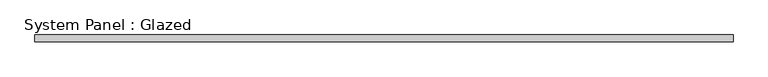
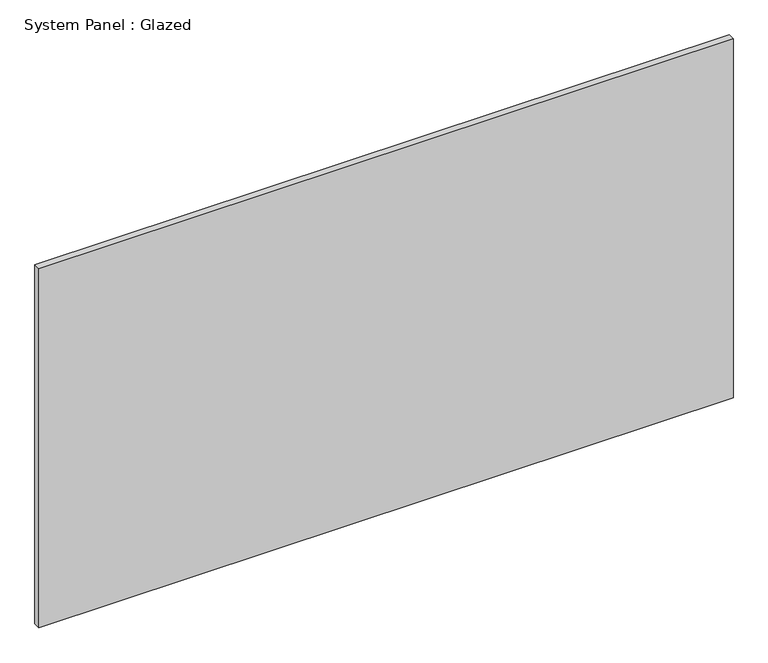
"""IFC4 building model written with IfcOpenShell, lengths in millimetres: plate geometry, System Panel : Glazed."""

from ifc_helpers import new_model, si_unit, origin, origin_with_axes, place, context, project, spatial, polyline, outline, extrude, source, transform, mapped, element, save


def system_panel_glazed_e2412059(model_context):
    return source(origin(), model_context, "Body", "SweptSolid", [
        extrude(outline(polyline([(1280.4735686, 19.05), (-1280.4735686, 19.05), (-1280.4735686, 44.45), (1280.4735686, 44.45), (1280.4735686, 19.05)])), origin_with_axes(), (0.0, 0.0, 1.0), 1400.215679),
    ])


if __name__ == "__main__":
    model = new_model("IFC4")
    model_context = context("Model", 3, world=origin())
    ifc_project = project(units=[si_unit("LENGTHUNIT", "METRE", prefix="MILLI")], contexts=[model_context])
    site = spatial("IfcSite", under=ifc_project)
    building = spatial("IfcBuilding", under=site)
    placement = place(None, origin())
    system_panel_glazed_shape = system_panel_glazed_e2412059(model_context)
    element("IfcPlate", 1, ObjectType="System Panel : Glazed", at=placement, inside=building, context=model_context, shape_type="MappedRepresentation", body=[
        mapped(system_panel_glazed_shape, transform((0.0, 0.0, 0.0), x_axis=(1.0, 0.0, 0.0), y_axis=(0.0, 1.0, 0.0), z_axis=(0.0, 0.0, 1.0))),
    ])
    save(model, "model.ifc")

# Revit data of these elements
# Type "System Panel : Glazed"
#   Construction Type Id = "GSP4R"
#   Analytic Construction = "1/8 in Pilkington single glazing"
#   Visual Light Transmittance = 0.9
#   Solar Heat Gain Coefficient = 0.86
#   Heat Transfer Coefficient (U) = 1.18115 BTU/(h·ft²·°F)
#   Define Thermal Properties by = 1
# Element 1 (IfcPlate, "System Panel : Glazed")
#   Materials on its faces: "Glass"
# Materials
#   "Glass": class "Glass", colour RGB 0 128 192, transparency 0.75, Description = "Soda Lime Glass", Cost = 0
